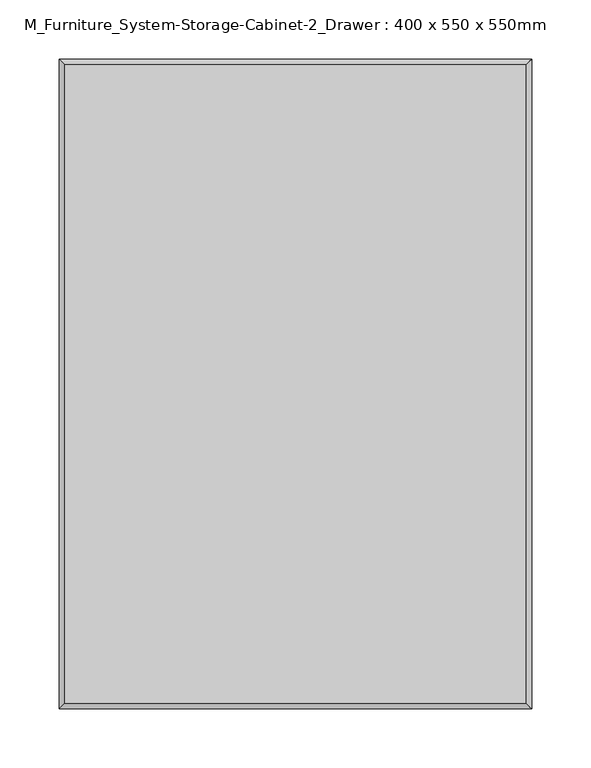
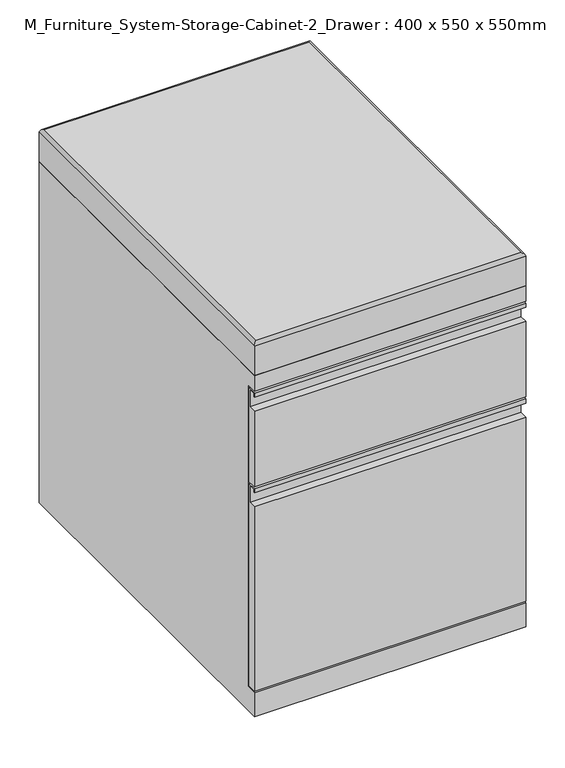
"""IFC4 building model written with IfcOpenShell, lengths in millimetres: furniture geometry, M_Furniture_System-Storage-Cabinet-2_Drawer : 400 x 550 x 550mm."""

from ifc_helpers import new_model, si_unit, frame, origin, place, context, project, spatial, polyline, ellipse_curve, outline, extrude, source, transform, mapped, element, save
from ifc_brep_helpers import plane_surface, cylinder_surface, advanced_brep


def m_furniture_system_storage_cabinet_2_drawer_400_x_550_x_4e0790d6(model_context):
    return source(origin(), model_context, "Body", "SolidModel", [
        extrude(outline(polyline([(0.0, 376.9625), (0.0, 494.8451302), (11.8998876, 494.8451302), (11.8998876, 521.4884893), (1.5239879, 521.4884893), (1.5239879, 516.6625121), (0.0, 516.6625121), (0.0, 523.0124879), (13.4873883, 523.0124879), (13.4873883, 376.9625), (0.0, 376.9625)])), frame((-200.0, 0.0, 0.0), z_axis=(1.0, 0.0, 0.0), x_axis=(0.0, 1.0, 0.0)), (0.0, 0.0, 1.0), 400.0),
        extrude(outline(polyline([(0.0, 58.7374985), (0.0, 345.6201544), (11.9293774, 345.6201544), (11.9293774, 372.2635136), (1.5239879, 372.2635136), (1.5239879, 367.4375), (0.0, 367.4375), (0.0, 373.7875121), (13.4873883, 373.7875121), (13.4873883, 58.7374985), (0.0, 58.7374985)])), frame((-200.0, 0.0, 0.0), z_axis=(1.0, 0.0, 0.0), x_axis=(0.0, 1.0, 0.0)), (0.0, 0.0, 1.0), 400.0),
        extrude(outline(polyline([(56.820048, 9.2063177), (51.9174039, 19.05), (100.4825718, 19.05), (95.5799278, 9.2063177), (86.9277397, 2.4185626), (76.1999879, 0.0), (65.4722406, 2.4185626), (56.820048, 9.2063177)])), frame((-146.025, 0.0, 0.0), z_axis=(1.0, 0.0, 0.0), x_axis=(0.0, 1.0, 0.0)), (0.0, 0.0, 1.0), 44.45),
        extrude(outline(polyline([(454.4200601, 9.2063177), (449.517416, 19.05), (498.082584, 19.05), (493.1799399, 9.2063177), (484.5277518, 2.4185626), (473.8, 0.0), (463.0722527, 2.4185626), (454.4200601, 9.2063177)])), frame((-146.025, 0.0, 0.0), z_axis=(1.0, 0.0, 0.0), x_axis=(0.0, 1.0, 0.0)), (0.0, 0.0, 1.0), 44.45),
        extrude(outline(polyline([(56.820048, 9.2063177), (51.9174039, 19.05), (100.4825718, 19.05), (95.5799278, 9.2063177), (86.9277397, 2.4185626), (76.1999879, 0.0), (65.4722406, 2.4185626), (56.820048, 9.2063177)])), frame((101.575, 0.0, 0.0), z_axis=(1.0, 0.0, 0.0), x_axis=(0.0, 1.0, 0.0)), (0.0, 0.0, 1.0), 44.45),
        extrude(outline(polyline([(498.082584, 19.05), (493.1799399, 9.2063177), (484.5277518, 2.4185626), (473.8, 0.0), (463.0722527, 2.4185626), (454.4200601, 9.2063177), (449.517416, 19.05), (498.082584, 19.05)])), frame((101.575, 0.0, 0.0), z_axis=(1.0, 0.0, 0.0), x_axis=(0.0, 1.0, 0.0)), (0.0, 0.0, 1.0), 44.45),
        extrude(outline(polyline([(0.0, 550.0), (550.0, 550.0), (550.0, 19.05), (0.0, 19.05), (0.0, 56.3562485), (16.6623883, 56.3562485), (16.6623883, 526.1875121), (0.0, 526.1875121), (0.0, 550.0)])), frame((-200.0, 0.0, 0.0), z_axis=(1.0, 0.0, 0.0), x_axis=(0.0, 1.0, 0.0)), (0.0, 0.0, 1.0), 400.0),
        advanced_brep(
        [(195.2375, 4.7625, 600.8), (195.2375, 545.2375, 600.8), (-195.2375, 545.2375, 600.8), (-195.2375, 4.7625, 600.8), (200.0, 550.0, 550.0), (200.0, 0.0, 550.0), (-200.0, 0.0, 550.0), (-200.0, 550.0, 550.0), (-200.0, 550.0, 596.0375), (200.0, 550.0, 596.0375), (-200.0, 0.0, 596.0375), (200.0, 0.0, 596.0375)],
        [
            (0, 1),
            (1, 2),
            (2, 3),
            (3, 0),
            (4, 5),
            (5, 6),
            (6, 7),
            (7, 4),
            (7, 8),
            (8, 9),
            (9, 4),
            (6, 10),
            (10, 8),
            (5, 11),
            (11, 10),
            (9, 11),
            (0, 11, ellipse_curve(frame((195.2375, 4.7625, 596.0375), z_axis=(0.7071067811865475, 0.7071067811865475, 0.0), x_axis=(0.7071067811865474, -0.7071067811865476, 0.0)), 6.7351921, 4.7625)),
            (9, 1, ellipse_curve(frame((195.2375, 545.2375, 596.0375), z_axis=(0.7071067811865475, -0.7071067811865475, 0.0), x_axis=(-0.7071067811865474, -0.7071067811865476, 0.0)), 6.7351921, 4.7625)),
            (3, 10, ellipse_curve(frame((-195.2375, 4.7625, 596.0375), z_axis=(0.7071067811865475, -0.7071067811865475, 0.0), x_axis=(-0.7071067811865476, -0.7071067811865474, 0.0)), 6.7351921, 4.7625)),
            (2, 8, ellipse_curve(frame((-195.2375, 545.2375, 596.0375), z_axis=(-0.7071067811865475, -0.7071067811865475, 0.0), x_axis=(-0.7071067811865474, 0.7071067811865476, 0.0)), 6.7351921, 4.7625)),
        ],
        [
            plane_surface(frame((-200.0, 550.0, 600.8), z_axis=(0.0, 0.0, 1.0), x_axis=(-1.0, 0.0, 0.0))),
            plane_surface(frame((-200.0, 550.0, 550.0), z_axis=(0.0, 0.0, -1.0), x_axis=(1.0, 0.0, 0.0))),
            plane_surface(frame((200.0, 550.0, 600.8), z_axis=(0.0, 1.0, 0.0), x_axis=(0.0, 0.0, -1.0))),
            plane_surface(frame((-200.0, 550.0, 600.8), z_axis=(-1.0, 0.0, 0.0), x_axis=(0.0, 0.0, -1.0))),
            plane_surface(frame((-200.0, 0.0, 600.8), z_axis=(0.0, -1.0, 0.0), x_axis=(0.0, 0.0, -1.0))),
            plane_surface(frame((200.0, 0.0, 600.8), z_axis=(1.0, 0.0, 0.0), x_axis=(0.0, 0.0, -1.0))),
            cylinder_surface(frame((195.2375, 550.0, 596.0375), z_axis=(0.0, -1.0, 0.0), x_axis=(1.0, 0.0, 0.0)), 4.7625),
            cylinder_surface(frame((200.0, 4.7625, 596.0375), z_axis=(-1.0, 0.0, 0.0), x_axis=(0.0, -1.0, 0.0)), 4.7625),
            cylinder_surface(frame((-195.2375, 0.0, 596.0375), z_axis=(0.0, 1.0, 0.0), x_axis=(-1.0, 0.0, 0.0)), 4.7625),
            cylinder_surface(frame((-200.0, 545.2375, 596.0375), z_axis=(1.0, 0.0, 0.0), x_axis=(0.0, 1.0, 0.0)), 4.7625),
        ],
        [
            (0, [[1, 2, 3, 4]]),
            (1, [[5, 6, 7, 8]]),
            (2, [[-8, 9, 10, 11]]),
            (3, [[-7, 12, 13, -9]]),
            (4, [[-6, 14, 15, -12]]),
            (5, [[-5, -11, 16, -14]]),
            (6, [[17, -16, 18, -1]]),
            (7, [[-17, -4, 19, -15]]),
            (8, [[-19, -3, 20, -13]]),
            (9, [[-18, -10, -20, -2]]),
        ],
    ),
    ])


if __name__ == "__main__":
    model = new_model("IFC4")
    model_context = context("Model", 3, world=origin())
    ifc_project = project(units=[si_unit("LENGTHUNIT", "METRE", prefix="MILLI")], contexts=[model_context])
    site = spatial("IfcSite", under=ifc_project)
    building = spatial("IfcBuilding", under=site)
    placement = place(None, origin())
    m_furniture_system_storage_cabinet_2_drawer_400_x_550_x_shape = m_furniture_system_storage_cabinet_2_drawer_400_x_550_x_4e0790d6(model_context)
    element("IfcFurniture", 1, ObjectType="M_Furniture_System-Storage-Cabinet-2_Drawer : 400 x 550 x 550mm", at=placement, inside=building, context=model_context, shape_type="MappedRepresentation", body=[
        mapped(m_furniture_system_storage_cabinet_2_drawer_400_x_550_x_shape, transform((0.0, 0.0, 0.0), x_axis=(1.0, 0.0, 0.0), y_axis=(0.0, 1.0, 0.0), z_axis=(0.0, 0.0, 1.0))),
    ])
    save(model, "model.ifc")

# Revit data of these elements
# Type "M_Furniture_System-Storage-Cabinet-2_Drawer : 400 x 550 x 550mm"
#   Type Comments = "400 x 550 x 550mm Double Drawer Cabinet"
#   Width = 400 mm
#   Height = 550 mm
#   Depth = 550 mm
#   Show Solid [instance default] = yes
#   Show Dashed [instance default] = no
#   Seat Visible [instance default] = yes
#   Drawer Material [instance default] = Metal - Paint - Beige
#   Cabinet Material [instance default] = Metal - Paint - Beige
#   Model = ""
#   Manufacturer = ""
#   Keynote = ""
#   Description = (empty or 0)
#   Default Elevation = 0
# Element 1 (IfcFurniture, "M_Furniture_System-Storage-Cabinet-2_Drawer : 400 x 550 x 550mm")
#   Materials on its faces: "Metal - Paint - Beige"
# Materials
#   "Metal - Paint - Beige": class "Metal", colour RGB 247 225 182, transparency 0
